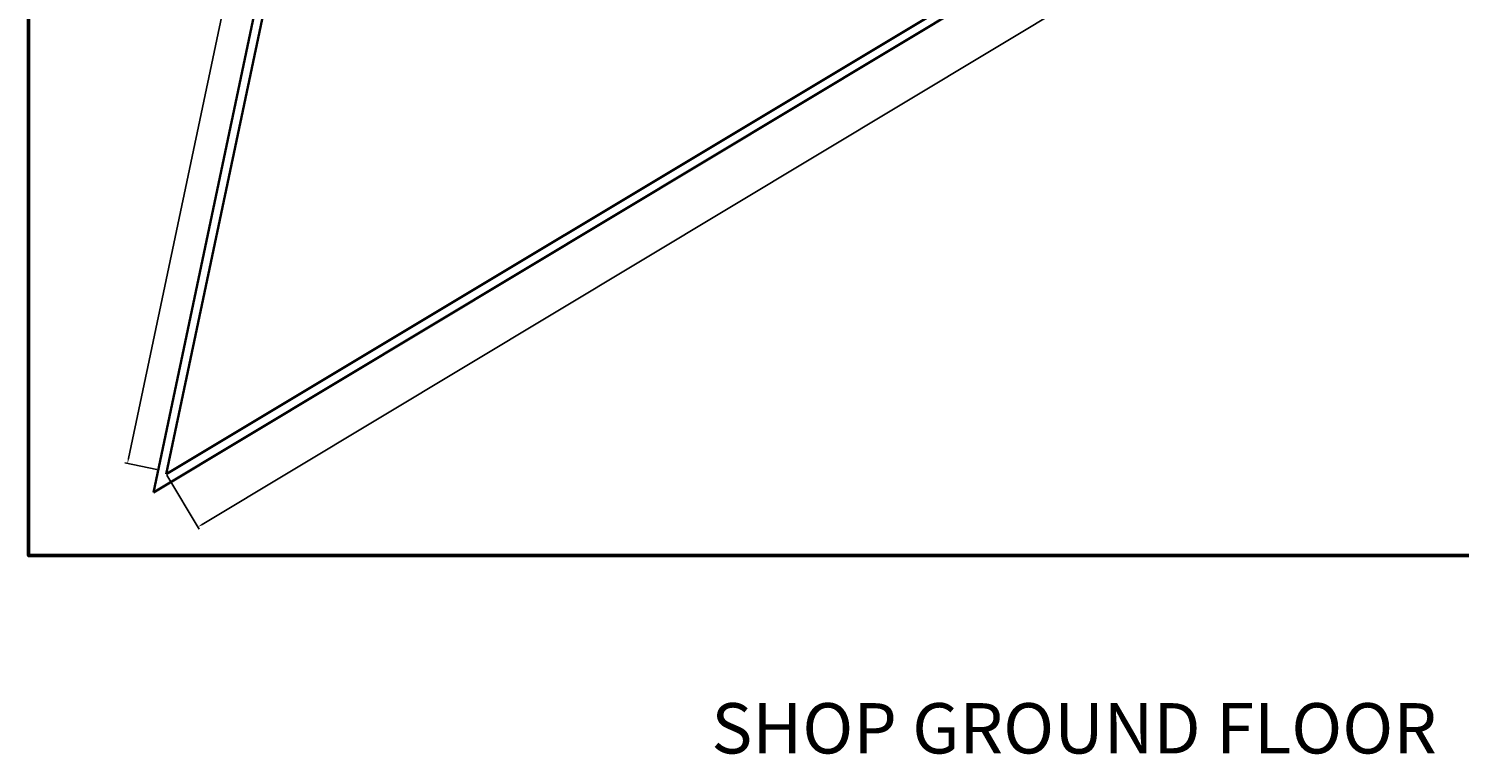
# Model space of a CAD drawing. Units: millimetres. Extents: x 2134 to 3363, y 1052 to 3233.
# Tile 1 of 11: x 2134 to 2854, y 1052 to 1417. Entities that reach past the tile are written whole.
import ezdxf

# ---------------------------------------------------------------- set-up
doc = ezdxf.new("R2010")
doc.units = ezdxf.units.MM
for name, color, linetype, lineweight in [('A-ANNO-DIMS', 2, 'Continuous', 18), ('A-ANNO-TTLB', 7, 'Continuous', 50), ('A-AREA-IDEN', 3, 'Continuous', 18), ('C-PROP', 6, 'Continuous', 35)]:
    doc.layers.add(name, color=color, linetype=linetype, lineweight=lineweight)
doc.styles.get("Standard").update_dxf_attribs({"font": 'arial.ttf'})
doc.styles.add('YQ_IDEN', font='COMPLEX.SHX', dxfattribs={"bigfont": 'GBCBIG.SHX'})
doc.dimstyles.new('ISO-25', dxfattribs={"dimtxt": 2.5, "dimasz": 2.5, "dimexe": 1.25, "dimexo": 0.625, "dimtad": 1, "dimtxsty": 'Standard', "dimcen": 2.5, "dimadec": 0, "dimazin": 0, "dimtfac": 1, "dimtmove": 0, "dimatfit": 3, "dimfxl": 1, "dimarcsym": 0})

# ---------------------------------------------------------------- blocks, each defined once
blk = doc.blocks.new('*D8')
at = {"layer": 'A-ANNO-DIMS', "color": 0, "lineweight": -2, "transparency": 16777216}
for p, q in [((2442.41, 2425.81), (2184.54, 1200.99)), ((2457.75, 2425.14), (2441.71, 2428.51)), ((2198.85, 1195.42), (2182.8, 1198.8))]:
    blk.add_line(p, q, dxfattribs=at)
at = {"layer": 'A-ANNO-DIMS', "color": 0, "transparency": 16777216}
for points in [[(2442.01, 2425.9), (2442.82, 2425.72), (2442.93, 2428.26)], [(2184.14, 1201.07), (2184.95, 1200.9), (2184.03, 1198.54)]]:
    blk.add_solid(points, dxfattribs=at)
at = {"layer": 'Defpoints', "color": 0, "transparency": 16777216}
for p in [(2458.36, 2425.01), (2184.03, 1198.54), (2199.46, 1195.29)]:
    blk.add_point(p, dxfattribs=at)
at = {"layer": 'A-ANNO-DIMS', "color": 0, "transparency": 16777216, "insert": (2311.4, 1813.84), "char_height": 2.5, "attachment_point": 5, "rotation": 78.11076}
blk.add_mtext('1256,67', dxfattribs=at)
blk = doc.blocks.new('*D10')
at = {"layer": 'A-ANNO-DIMS', "color": 0, "lineweight": -2, "transparency": 16777216}
for p, q in [((3164.66, 1769.83), (3180.9, 1742.8)), ((3178.12, 1742.58), (2221.66, 1167.89)), ((2203.92, 1192.56), (2220.16, 1165.53))]:
    blk.add_line(p, q, dxfattribs=at)
at = {"layer": 'A-ANNO-DIMS', "color": 0, "transparency": 16777216}
for points in [[(3177.9, 1742.94), (3178.33, 1742.23), (3180.26, 1743.87)], [(2221.44, 1168.24), (2221.87, 1167.53), (2219.52, 1166.6)]]:
    blk.add_solid(points, dxfattribs=at)
at = {"layer": 'Defpoints', "color": 0, "transparency": 16777216}
for p in [(3164.34, 1770.37), (2203.6, 1193.09), (2219.52, 1166.6)]:
    blk.add_point(p, dxfattribs=at)
at = {"layer": 'A-ANNO-DIMS', "color": 0, "transparency": 16777216, "insert": (2674.71, 1442.59), "char_height": 2.5, "attachment_point": 5, "rotation": 31}
blk.add_mtext('1120,83', dxfattribs=at)
blk = doc.blocks.new('*D6')
at = {"layer": 'A-ANNO-DIMS', "color": 0, "lineweight": -2, "transparency": 16777216}
blk.add_arc((2458.36, 2425.01), 20.29, 94.06404, 251.04672, dxfattribs=at)
at = {"layer": 'A-ANNO-DIMS', "color": 0, "transparency": 16777216}
for points in [[(2456.92, 2445.66), (2456.93, 2444.83), (2459.42, 2445.27)], [(2451.88, 2406.22), (2451.66, 2405.42), (2454.18, 2405.15)]]:
    blk.add_solid(points, dxfattribs=at)
at = {"layer": 'Defpoints', "color": 0, "transparency": 16777216}
for p in [(2491.84, 3063.82), (2441.94, 2436.92), (2458.36, 2425.01), (2458.36, 2425.01), (2197.07, 1183.92)]:
    blk.add_point(p, dxfattribs=at)
at = {"layer": 'A-ANNO-DIMS', "color": 0, "transparency": 16777216, "insert": (2436.38, 2427.88), "char_height": 2.5, "attachment_point": 5, "rotation": 82.55538}
blk.add_mtext('171°', dxfattribs=at)

msp = doc.modelspace()

# ---------------------------------------------------------------- linework, layer by layer
at = {"layer": 'A-ANNO-TTLB', "ltscale": 0.5}
msp.add_lwpolyline([(2134.34, 3233.23), (3362.77, 3233.23), (3362.77, 1152.237), (2134.34, 1152.237)], close=True, dxfattribs=at)
at = {"layer": 'C-PROP'}
for p, q in [((2197.066, 1183.92), (2458.361, 2425.007)), ((2203.596, 1193.093), (2462.764, 2424.08)), ((3164.339, 1770.366), (2203.596, 1193.093)), ((3168.839, 1767.82), (2197.066, 1183.92))]:
    msp.add_line(p, q, dxfattribs=at)

# ---------------------------------------------------------------- texts
at = {"layer": 'A-AREA-IDEN', "ltscale": 0.5, "insert": (2477.721, 1077.997), "char_height": 25.33, "attachment_point": 1, "style": 'YQ_IDEN'}
msp.add_mtext_dynamic_manual_height_columns('SHOP GROUND FLOOR', width=658.32978, gutter_width=12.5, heights=[0], dxfattribs=at)

# ---------------------------------------------------------------- dimensions: what is measured, and where the dimension line sits
at = {"layer": 'A-ANNO-DIMS'}
dim = msp.add_angular_dim_2l(base=(2441.938, 2436.923), line1=((2197.066, 1183.92), (2458.361, 2425.007)), line2=((2458.361, 2425.007), (2491.839, 3063.82)), dimstyle='ISO-25', override={"dimclrd": 0, "dimclre": 0, "dimclrt": 0}, dxfattribs=at)
dim.commit()
dim.dimension.update_dxf_attribs({"geometry": '*D6', "text_midpoint": (2436.377, 2427.88)})
dim = msp.add_aligned_dim(p1=(2458.361, 2425.007), p2=(2199.46, 1195.291), distance=-15.77, dimstyle='ISO-25', override={"dimclrd": 0, "dimclre": 0, "dimclrt": 0}, dxfattribs=at)
dim.commit()
dim.dimension.update_dxf_attribs({"geometry": '*D8', "text_midpoint": (2311.397, 1813.836)})
dim = msp.add_linear_dim(base=(2219.5153, 1166.599), p1=(3164.339, 1770.3661), p2=(2203.5959, 1193.0934), angle=211, dimstyle='ISO-25', override={"dimclrd": 0, "dimclre": 0, "dimclrt": 0}, dxfattribs=at)
dim.commit()
dim.dimension.update_dxf_attribs({"geometry": '*D10', "text_midpoint": (2675.8085, 1440.7677), "dimtype": 161})

doc.saveas('drawing.dxf')
